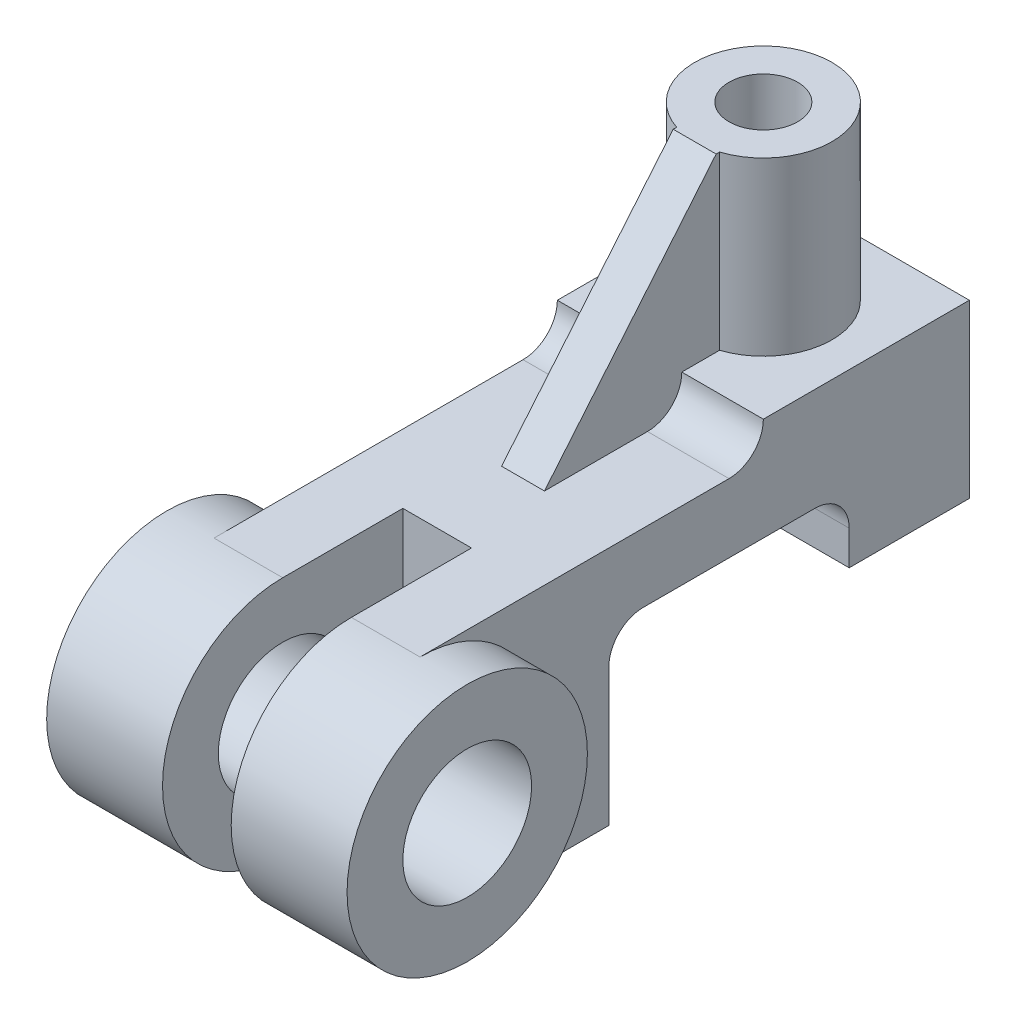
ISO-10303-21;
HEADER;
FILE_DESCRIPTION(('STEP AP214'),'2;1');
FILE_NAME('part.step','',(''),(''),'','','');
FILE_SCHEMA(('AUTOMOTIVE_DESIGN { 1 0 10303 214 1 1 1 1 }'));
ENDSEC;
DATA;
#1=APPLICATION_CONTEXT('core data for automotive mechanical design processes');
#2=APPLICATION_PROTOCOL_DEFINITION('international standard','automotive_design',2000,#1);
#3=PRODUCT_CONTEXT('',#1,'mechanical');
#4=PRODUCT('Part','Part','',(#3));
#5=PRODUCT_RELATED_PRODUCT_CATEGORY('part','',(#4));
#6=PRODUCT_DEFINITION_FORMATION('','',#4);
#7=PRODUCT_DEFINITION_CONTEXT('part definition',#1,'design');
#8=PRODUCT_DEFINITION('design','',#6,#7);
#9=PRODUCT_DEFINITION_SHAPE('','',#8);
#10=(LENGTH_UNIT() NAMED_UNIT(*) SI_UNIT(.MILLI.,.METRE.));
#11=(NAMED_UNIT(*) PLANE_ANGLE_UNIT() SI_UNIT($,.RADIAN.));
#12=(NAMED_UNIT(*) SI_UNIT($,.STERADIAN.) SOLID_ANGLE_UNIT());
#13=UNCERTAINTY_MEASURE_WITH_UNIT(LENGTH_MEASURE(1.E-05),#10,'distance_accuracy_value','');
#14=(GEOMETRIC_REPRESENTATION_CONTEXT(3) GLOBAL_UNCERTAINTY_ASSIGNED_CONTEXT((#13)) GLOBAL_UNIT_ASSIGNED_CONTEXT((#10,
#11,#12)) REPRESENTATION_CONTEXT('',''));
#15=CARTESIAN_POINT('',(0.,0.,0.));
#16=DIRECTION('',(0.,0.,1.));
#17=DIRECTION('',(1.,0.,0.));
#18=AXIS2_PLACEMENT_3D('',#15,#16,#17);
#19=CARTESIAN_POINT('',(24.,36.,-72.));
#20=DIRECTION('',(1.,0.,0.));
#21=DIRECTION('',(0.,0.,-1.));
#22=AXIS2_PLACEMENT_3D('',#19,#20,#21);
#23=CYLINDRICAL_SURFACE('',#22,8.);
#24=CARTESIAN_POINT('',(-5.,36.,-72.));
#25=DIRECTION('',(1.,0.,0.));
#26=DIRECTION('',(0.,0.,-1.));
#27=AXIS2_PLACEMENT_3D('',#24,#25,#26);
#28=CIRCLE('',#27,8.);
#29=CARTESIAN_POINT('',(-5.,36.,-80.));
#30=VERTEX_POINT('',#29);
#31=CARTESIAN_POINT('',(-5.,28.,-72.));
#32=VERTEX_POINT('',#31);
#33=EDGE_CURVE('E229',#30,#32,#28,.F.);
#34=ORIENTED_EDGE('',*,*,#33,.F.);
#35=DIRECTION('',(-1.,0.,0.));
#36=VECTOR('',#35,1.);
#37=CARTESIAN_POINT('',(24.,36.,-80.));
#38=LINE('',#37,#36);
#39=CARTESIAN_POINT('',(-24.,36.,-80.));
#40=VERTEX_POINT('',#39);
#41=EDGE_CURVE('E335',#30,#40,#38,.T.);
#42=ORIENTED_EDGE('',*,*,#41,.T.);
#43=CARTESIAN_POINT('',(-24.,36.,-72.));
#44=DIRECTION('',(1.,0.,0.));
#45=DIRECTION('',(0.,0.,-1.));
#46=AXIS2_PLACEMENT_3D('',#43,#44,#45);
#47=CIRCLE('',#46,8.);
#48=CARTESIAN_POINT('',(-24.,28.,-72.));
#49=VERTEX_POINT('',#48);
#50=EDGE_CURVE('E383',#49,#40,#47,.T.);
#51=ORIENTED_EDGE('',*,*,#50,.F.);
#52=DIRECTION('',(-1.,0.,0.));
#53=VECTOR('',#52,1.);
#54=CARTESIAN_POINT('',(-24.,28.,-72.));
#55=LINE('',#54,#53);
#56=EDGE_CURVE('E374',#32,#49,#55,.T.);
#57=ORIENTED_EDGE('',*,*,#56,.F.);
#58=EDGE_LOOP('',(#34,#42,#51,#57));
#59=FACE_BOUND('',#58,.T.);
#60=ADVANCED_FACE('F52',(#59),#23,.F.);
#61=CARTESIAN_POINT('',(35.,0.,0.));
#62=DIRECTION('',(-1.,0.,0.));
#63=DIRECTION('',(0.,0.,1.));
#64=AXIS2_PLACEMENT_3D('',#61,#62,#63);
#65=CYLINDRICAL_SURFACE('',#64,28.);
#66=CARTESIAN_POINT('',(-35.,0.,0.));
#67=DIRECTION('',(1.,0.,0.));
#68=DIRECTION('',(0.,0.,-1.));
#69=AXIS2_PLACEMENT_3D('',#66,#67,#68);
#70=CIRCLE('',#69,28.);
#71=CARTESIAN_POINT('',(-35.,0.,-28.));
#72=VERTEX_POINT('',#71);
#73=EDGE_CURVE('E355',#72,#72,#70,.T.);
#74=ORIENTED_EDGE('',*,*,#73,.T.);
#75=EDGE_LOOP('',(#74));
#76=FACE_BOUND('',#75,.T.);
#77=CARTESIAN_POINT('',(-7.99999999999999,0.,0.));
#78=DIRECTION('',(-1.,0.,0.));
#79=DIRECTION('',(0.,0.,1.));
#80=AXIS2_PLACEMENT_3D('',#77,#78,#79);
#81=CIRCLE('',#80,28.);
#82=CARTESIAN_POINT('',(-8.,-28.,0.));
#83=VERTEX_POINT('',#82);
#84=CARTESIAN_POINT('',(-8.,28.,0.));
#85=VERTEX_POINT('',#84);
#86=EDGE_CURVE('E272',#83,#85,#81,.T.);
#87=ORIENTED_EDGE('',*,*,#86,.T.);
#88=DIRECTION('',(-1.,0.,0.));
#89=VECTOR('',#88,1.);
#90=CARTESIAN_POINT('',(24.,28.,0.));
#91=LINE('',#90,#89);
#92=CARTESIAN_POINT('',(-24.,28.,0.));
#93=VERTEX_POINT('',#92);
#94=EDGE_CURVE('E303',#85,#93,#91,.T.);
#95=ORIENTED_EDGE('',*,*,#94,.T.);
#96=CARTESIAN_POINT('',(-24.,0.,0.));
#97=DIRECTION('',(1.,0.,0.));
#98=DIRECTION('',(0.,0.,-1.));
#99=AXIS2_PLACEMENT_3D('',#96,#97,#98);
#100=CIRCLE('',#99,28.);
#101=CARTESIAN_POINT('',(-24.,-28.,0.));
#102=VERTEX_POINT('',#101);
#103=EDGE_CURVE('E278',#102,#93,#100,.T.);
#104=ORIENTED_EDGE('',*,*,#103,.F.);
#105=DIRECTION('',(-1.,0.,0.));
#106=VECTOR('',#105,1.);
#107=CARTESIAN_POINT('',(24.,-28.,0.));
#108=LINE('',#107,#106);
#109=EDGE_CURVE('E345',#83,#102,#108,.T.);
#110=ORIENTED_EDGE('',*,*,#109,.F.);
#111=EDGE_LOOP('',(#87,#95,#104,#110));
#112=FACE_BOUND('',#111,.T.);
#113=ADVANCED_FACE('F422',(#76,#112),#65,.T.);
#114=CARTESIAN_POINT('',(35.,0.,0.));
#115=DIRECTION('',(-1.,0.,0.));
#116=DIRECTION('',(0.,0.,1.));
#117=AXIS2_PLACEMENT_3D('',#114,#115,#116);
#118=CYLINDRICAL_SURFACE('',#117,15.);
#119=CARTESIAN_POINT('',(-7.99999999999999,0.,0.));
#120=DIRECTION('',(-1.,0.,0.));
#121=DIRECTION('',(0.,0.,1.));
#122=AXIS2_PLACEMENT_3D('',#119,#120,#121);
#123=CIRCLE('',#122,15.);
#124=CARTESIAN_POINT('',(-7.99999999999999,0.,15.));
#125=VERTEX_POINT('',#124);
#126=EDGE_CURVE('E271',#125,#125,#123,.T.);
#127=ORIENTED_EDGE('',*,*,#126,.F.);
#128=EDGE_LOOP('',(#127));
#129=FACE_BOUND('',#128,.T.);
#130=CARTESIAN_POINT('',(-35.,0.,0.));
#131=DIRECTION('',(1.,0.,0.));
#132=DIRECTION('',(0.,0.,-1.));
#133=AXIS2_PLACEMENT_3D('',#130,#131,#132);
#134=CIRCLE('',#133,15.);
#135=CARTESIAN_POINT('',(-35.,0.,-15.));
#136=VERTEX_POINT('',#135);
#137=EDGE_CURVE('E348',#136,#136,#134,.T.);
#138=ORIENTED_EDGE('',*,*,#137,.F.);
#139=EDGE_LOOP('',(#138));
#140=FACE_BOUND('',#139,.T.);
#141=ADVANCED_FACE('F487',(#129,#140),#118,.F.);
#142=CARTESIAN_POINT('',(24.,-28.,0.));
#143=DIRECTION('',(0.,-1.,0.));
#144=DIRECTION('',(0.,0.,-1.));
#145=AXIS2_PLACEMENT_3D('',#142,#143,#144);
#146=PLANE('',#145);
#147=DIRECTION('',(-1.,0.,0.));
#148=VECTOR('',#147,1.);
#149=CARTESIAN_POINT('',(-8.,-28.,-28.));
#150=LINE('',#149,#148);
#151=CARTESIAN_POINT('',(8.,-28.,-28.));
#152=VERTEX_POINT('',#151);
#153=CARTESIAN_POINT('',(-8.,-28.,-28.));
#154=VERTEX_POINT('',#153);
#155=EDGE_CURVE('E257',#152,#154,#150,.T.);
#156=ORIENTED_EDGE('',*,*,#155,.T.);
#157=DIRECTION('',(0.,0.,1.));
#158=VECTOR('',#157,1.);
#159=CARTESIAN_POINT('',(-8.,-28.,-28.));
#160=LINE('',#159,#158);
#161=EDGE_CURVE('E252',#154,#83,#160,.T.);
#162=ORIENTED_EDGE('',*,*,#161,.T.);
#163=ORIENTED_EDGE('',*,*,#109,.T.);
#164=DIRECTION('',(0.,0.,1.));
#165=VECTOR('',#164,1.);
#166=CARTESIAN_POINT('',(-24.,-28.,0.));
#167=LINE('',#166,#165);
#168=CARTESIAN_POINT('',(-24.,-28.,-44.));
#169=VERTEX_POINT('',#168);
#170=EDGE_CURVE('E306',#169,#102,#167,.T.);
#171=ORIENTED_EDGE('',*,*,#170,.F.);
#172=DIRECTION('',(-1.,0.,0.));
#173=VECTOR('',#172,1.);
#174=CARTESIAN_POINT('',(24.,-28.,-44.));
#175=LINE('',#174,#173);
#176=CARTESIAN_POINT('',(24.,-28.,-44.));
#177=VERTEX_POINT('',#176);
#178=EDGE_CURVE('E344',#177,#169,#175,.T.);
#179=ORIENTED_EDGE('',*,*,#178,.F.);
#180=DIRECTION('',(0.,0.,1.));
#181=VECTOR('',#180,1.);
#182=CARTESIAN_POINT('',(24.,-28.,0.));
#183=LINE('',#182,#181);
#184=CARTESIAN_POINT('',(24.,-28.,0.));
#185=VERTEX_POINT('',#184);
#186=EDGE_CURVE('E280',#177,#185,#183,.T.);
#187=ORIENTED_EDGE('',*,*,#186,.T.);
#188=CARTESIAN_POINT('',(8.,-28.,0.));
#189=VERTEX_POINT('',#188);
#190=EDGE_CURVE('E341',#185,#189,#108,.T.);
#191=ORIENTED_EDGE('',*,*,#190,.T.);
#192=DIRECTION('',(0.,0.,-1.));
#193=VECTOR('',#192,1.);
#194=CARTESIAN_POINT('',(8.,-28.,-28.));
#195=LINE('',#194,#193);
#196=EDGE_CURVE('E253',#189,#152,#195,.T.);
#197=ORIENTED_EDGE('',*,*,#196,.T.);
#198=EDGE_LOOP('',(#156,#162,#163,#171,#179,#187,#191,#197));
#199=FACE_BOUND('',#198,.T.);
#200=ADVANCED_FACE('F439',(#199),#146,.T.);
#201=CARTESIAN_POINT('',(24.,28.,0.));
#202=VERTEX_POINT('',#201);
#203=CARTESIAN_POINT('',(8.,28.,0.));
#204=VERTEX_POINT('',#203);
#205=EDGE_CURVE('E329',#202,#204,#91,.T.);
#206=ORIENTED_EDGE('',*,*,#205,.T.);
#207=CARTESIAN_POINT('',(8.,0.,0.));
#208=DIRECTION('',(1.,0.,0.));
#209=DIRECTION('',(0.,0.,-1.));
#210=AXIS2_PLACEMENT_3D('',#207,#208,#209);
#211=CIRCLE('',#210,28.);
#212=EDGE_CURVE('E264',#204,#189,#211,.T.);
#213=ORIENTED_EDGE('',*,*,#212,.T.);
#214=ORIENTED_EDGE('',*,*,#190,.F.);
#215=CARTESIAN_POINT('',(24.,0.,0.));
#216=DIRECTION('',(1.,0.,0.));
#217=DIRECTION('',(0.,0.,-1.));
#218=AXIS2_PLACEMENT_3D('',#215,#216,#217);
#219=CIRCLE('',#218,28.);
#220=EDGE_CURVE('E279',#185,#202,#219,.T.);
#221=ORIENTED_EDGE('',*,*,#220,.T.);
#222=EDGE_LOOP('',(#206,#213,#214,#221));
#223=FACE_BOUND('',#222,.T.);
#224=CARTESIAN_POINT('',(35.,0.,0.));
#225=DIRECTION('',(1.,0.,0.));
#226=DIRECTION('',(0.,0.,-1.));
#227=AXIS2_PLACEMENT_3D('',#224,#225,#226);
#228=CIRCLE('',#227,28.);
#229=CARTESIAN_POINT('',(35.,0.,-28.));
#230=VERTEX_POINT('',#229);
#231=EDGE_CURVE('E354',#230,#230,#228,.T.);
#232=ORIENTED_EDGE('',*,*,#231,.F.);
#233=EDGE_LOOP('',(#232));
#234=FACE_BOUND('',#233,.T.);
#235=ADVANCED_FACE('F433',(#223,#234),#65,.T.);
#236=CARTESIAN_POINT('',(35.,0.,0.));
#237=DIRECTION('',(1.,0.,0.));
#238=DIRECTION('',(0.,0.,-1.));
#239=AXIS2_PLACEMENT_3D('',#236,#237,#238);
#240=PLANE('',#239);
#241=ORIENTED_EDGE('',*,*,#231,.T.);
#242=EDGE_LOOP('',(#241));
#243=FACE_BOUND('',#242,.T.);
#244=CARTESIAN_POINT('',(35.,0.,0.));
#245=DIRECTION('',(1.,0.,0.));
#246=DIRECTION('',(0.,0.,-1.));
#247=AXIS2_PLACEMENT_3D('',#244,#245,#246);
#248=CIRCLE('',#247,15.);
#249=CARTESIAN_POINT('',(35.,0.,-15.));
#250=VERTEX_POINT('',#249);
#251=EDGE_CURVE('E349',#250,#250,#248,.T.);
#252=ORIENTED_EDGE('',*,*,#251,.F.);
#253=EDGE_LOOP('',(#252));
#254=FACE_BOUND('',#253,.T.);
#255=ADVANCED_FACE('F503',(#243,#254),#240,.T.);
#256=CARTESIAN_POINT('',(-35.,0.,0.));
#257=DIRECTION('',(1.,0.,0.));
#258=DIRECTION('',(0.,0.,-1.));
#259=AXIS2_PLACEMENT_3D('',#256,#257,#258);
#260=PLANE('',#259);
#261=ORIENTED_EDGE('',*,*,#73,.F.);
#262=EDGE_LOOP('',(#261));
#263=FACE_BOUND('',#262,.T.);
#264=ORIENTED_EDGE('',*,*,#137,.T.);
#265=EDGE_LOOP('',(#264));
#266=FACE_BOUND('',#265,.T.);
#267=ADVANCED_FACE('F502',(#263,#266),#260,.F.);
#268=CARTESIAN_POINT('',(8.,0.,0.));
#269=DIRECTION('',(1.,0.,0.));
#270=DIRECTION('',(0.,0.,-1.));
#271=AXIS2_PLACEMENT_3D('',#268,#269,#270);
#272=CIRCLE('',#271,15.);
#273=CARTESIAN_POINT('',(8.,0.,-15.));
#274=VERTEX_POINT('',#273);
#275=EDGE_CURVE('E267',#274,#274,#272,.T.);
#276=ORIENTED_EDGE('',*,*,#275,.F.);
#277=EDGE_LOOP('',(#276));
#278=FACE_BOUND('',#277,.T.);
#279=ORIENTED_EDGE('',*,*,#251,.T.);
#280=EDGE_LOOP('',(#279));
#281=FACE_BOUND('',#280,.T.);
#282=ADVANCED_FACE('F510',(#278,#281),#118,.F.);
#283=CARTESIAN_POINT('',(24.,0.,-44.));
#284=DIRECTION('',(0.,0.,-1.));
#285=DIRECTION('',(0.,1.,0.));
#286=AXIS2_PLACEMENT_3D('',#283,#284,#285);
#287=PLANE('',#286);
#288=ORIENTED_EDGE('',*,*,#178,.T.);
#289=DIRECTION('',(0.,-1.,0.));
#290=VECTOR('',#289,1.);
#291=CARTESIAN_POINT('',(-24.,0.,-44.));
#292=LINE('',#291,#290);
#293=CARTESIAN_POINT('',(-24.,3.99999999999999,-44.));
#294=VERTEX_POINT('',#293);
#295=EDGE_CURVE('E307',#294,#169,#292,.T.);
#296=ORIENTED_EDGE('',*,*,#295,.F.);
#297=DIRECTION('',(-1.,0.,0.));
#298=VECTOR('',#297,1.);
#299=CARTESIAN_POINT('',(24.,3.99999999999999,-44.));
#300=LINE('',#299,#298);
#301=CARTESIAN_POINT('',(24.,3.99999999999999,-44.));
#302=VERTEX_POINT('',#301);
#303=EDGE_CURVE('E373',#294,#302,#300,.F.);
#304=ORIENTED_EDGE('',*,*,#303,.T.);
#305=DIRECTION('',(0.,-1.,0.));
#306=VECTOR('',#305,1.);
#307=CARTESIAN_POINT('',(24.,0.,-44.));
#308=LINE('',#307,#306);
#309=EDGE_CURVE('E283',#302,#177,#308,.T.);
#310=ORIENTED_EDGE('',*,*,#309,.T.);
#311=EDGE_LOOP('',(#288,#296,#304,#310));
#312=FACE_BOUND('',#311,.T.);
#313=ADVANCED_FACE('F443',(#312),#287,.T.);
#314=CARTESIAN_POINT('',(24.,12.,0.));
#315=DIRECTION('',(0.,-1.,0.));
#316=DIRECTION('',(0.,0.,-1.));
#317=AXIS2_PLACEMENT_3D('',#314,#315,#316);
#318=PLANE('',#317);
#319=DIRECTION('',(-1.,0.,0.));
#320=VECTOR('',#319,1.);
#321=CARTESIAN_POINT('',(-24.,12.,-52.));
#322=LINE('',#321,#320);
#323=CARTESIAN_POINT('',(24.,12.,-52.));
#324=VERTEX_POINT('',#323);
#325=CARTESIAN_POINT('',(-24.,12.,-52.));
#326=VERTEX_POINT('',#325);
#327=EDGE_CURVE('E367',#324,#326,#322,.T.);
#328=ORIENTED_EDGE('',*,*,#327,.T.);
#329=DIRECTION('',(0.,0.,1.));
#330=VECTOR('',#329,1.);
#331=CARTESIAN_POINT('',(-24.,12.,0.));
#332=LINE('',#331,#330);
#333=CARTESIAN_POINT('',(-24.,12.,-92.));
#334=VERTEX_POINT('',#333);
#335=EDGE_CURVE('E315',#334,#326,#332,.T.);
#336=ORIENTED_EDGE('',*,*,#335,.F.);
#337=DIRECTION('',(-1.,0.,0.));
#338=VECTOR('',#337,1.);
#339=CARTESIAN_POINT('',(24.,12.,-92.));
#340=LINE('',#339,#338);
#341=CARTESIAN_POINT('',(24.,12.,-92.));
#342=VERTEX_POINT('',#341);
#343=EDGE_CURVE('E371',#334,#342,#340,.F.);
#344=ORIENTED_EDGE('',*,*,#343,.T.);
#345=DIRECTION('',(0.,0.,1.));
#346=VECTOR('',#345,1.);
#347=CARTESIAN_POINT('',(24.,12.,0.));
#348=LINE('',#347,#346);
#349=EDGE_CURVE('E281',#342,#324,#348,.T.);
#350=ORIENTED_EDGE('',*,*,#349,.T.);
#351=EDGE_LOOP('',(#328,#336,#344,#350));
#352=FACE_BOUND('',#351,.T.);
#353=ADVANCED_FACE('F451',(#352),#318,.T.);
#354=CARTESIAN_POINT('',(24.,0.,-100.));
#355=DIRECTION('',(0.,0.,1.));
#356=DIRECTION('',(1.,0.,0.));
#357=AXIS2_PLACEMENT_3D('',#354,#355,#356);
#358=PLANE('',#357);
#359=DIRECTION('',(-1.,0.,0.));
#360=VECTOR('',#359,1.);
#361=CARTESIAN_POINT('',(-24.,4.,-100.));
#362=LINE('',#361,#360);
#363=CARTESIAN_POINT('',(24.,4.,-100.));
#364=VERTEX_POINT('',#363);
#365=CARTESIAN_POINT('',(-24.,4.,-100.));
#366=VERTEX_POINT('',#365);
#367=EDGE_CURVE('E370',#364,#366,#362,.T.);
#368=ORIENTED_EDGE('',*,*,#367,.T.);
#369=DIRECTION('',(0.,1.,0.));
#370=VECTOR('',#369,1.);
#371=CARTESIAN_POINT('',(-24.,0.,-100.));
#372=LINE('',#371,#370);
#373=CARTESIAN_POINT('',(-24.,-4.,-100.));
#374=VERTEX_POINT('',#373);
#375=EDGE_CURVE('E314',#374,#366,#372,.T.);
#376=ORIENTED_EDGE('',*,*,#375,.F.);
#377=DIRECTION('',(-1.,0.,0.));
#378=VECTOR('',#377,1.);
#379=CARTESIAN_POINT('',(24.,-4.,-100.));
#380=LINE('',#379,#378);
#381=CARTESIAN_POINT('',(24.,-4.,-100.));
#382=VERTEX_POINT('',#381);
#383=EDGE_CURVE('E338',#382,#374,#380,.T.);
#384=ORIENTED_EDGE('',*,*,#383,.F.);
#385=DIRECTION('',(0.,1.,0.));
#386=VECTOR('',#385,1.);
#387=CARTESIAN_POINT('',(24.,0.,-100.));
#388=LINE('',#387,#386);
#389=EDGE_CURVE('E287',#382,#364,#388,.T.);
#390=ORIENTED_EDGE('',*,*,#389,.T.);
#391=EDGE_LOOP('',(#368,#376,#384,#390));
#392=FACE_BOUND('',#391,.T.);
#393=ADVANCED_FACE('F463',(#392),#358,.T.);
#394=CARTESIAN_POINT('',(24.,-4.00000000000001,0.));
#395=DIRECTION('',(0.,-1.,0.));
#396=DIRECTION('',(0.,0.,-1.));
#397=AXIS2_PLACEMENT_3D('',#394,#395,#396);
#398=PLANE('',#397);
#399=ORIENTED_EDGE('',*,*,#383,.T.);
#400=DIRECTION('',(0.,0.,1.));
#401=VECTOR('',#400,1.);
#402=CARTESIAN_POINT('',(-24.,-4.00000000000001,0.));
#403=LINE('',#402,#401);
#404=CARTESIAN_POINT('',(-24.,-4.,-128.));
#405=VERTEX_POINT('',#404);
#406=EDGE_CURVE('E319',#405,#374,#403,.T.);
#407=ORIENTED_EDGE('',*,*,#406,.F.);
#408=DIRECTION('',(-1.,0.,0.));
#409=VECTOR('',#408,1.);
#410=CARTESIAN_POINT('',(24.,-4.,-128.));
#411=LINE('',#410,#409);
#412=CARTESIAN_POINT('',(24.,-4.,-128.));
#413=VERTEX_POINT('',#412);
#414=EDGE_CURVE('E336',#413,#405,#411,.T.);
#415=ORIENTED_EDGE('',*,*,#414,.F.);
#416=DIRECTION('',(0.,0.,1.));
#417=VECTOR('',#416,1.);
#418=CARTESIAN_POINT('',(24.,-4.00000000000001,0.));
#419=LINE('',#418,#417);
#420=EDGE_CURVE('E293',#413,#382,#419,.T.);
#421=ORIENTED_EDGE('',*,*,#420,.T.);
#422=EDGE_LOOP('',(#399,#407,#415,#421));
#423=FACE_BOUND('',#422,.T.);
#424=ADVANCED_FACE('F466',(#423),#398,.T.);
#425=CARTESIAN_POINT('',(24.,0.,-128.));
#426=DIRECTION('',(0.,0.,-1.));
#427=DIRECTION('',(-1.,0.,0.));
#428=AXIS2_PLACEMENT_3D('',#425,#426,#427);
#429=PLANE('',#428);
#430=ORIENTED_EDGE('',*,*,#414,.T.);
#431=DIRECTION('',(0.,-1.,0.));
#432=VECTOR('',#431,1.);
#433=CARTESIAN_POINT('',(-24.,0.,-128.));
#434=LINE('',#433,#432);
#435=CARTESIAN_POINT('',(-24.,36.,-128.));
#436=VERTEX_POINT('',#435);
#437=EDGE_CURVE('E323',#436,#405,#434,.T.);
#438=ORIENTED_EDGE('',*,*,#437,.F.);
#439=DIRECTION('',(-1.,0.,0.));
#440=VECTOR('',#439,1.);
#441=CARTESIAN_POINT('',(24.,36.,-128.));
#442=LINE('',#441,#440);
#443=CARTESIAN_POINT('',(24.,36.,-128.));
#444=VERTEX_POINT('',#443);
#445=EDGE_CURVE('E337',#444,#436,#442,.T.);
#446=ORIENTED_EDGE('',*,*,#445,.F.);
#447=DIRECTION('',(0.,-1.,0.));
#448=VECTOR('',#447,1.);
#449=CARTESIAN_POINT('',(24.,0.,-128.));
#450=LINE('',#449,#448);
#451=EDGE_CURVE('E295',#444,#413,#450,.T.);
#452=ORIENTED_EDGE('',*,*,#451,.T.);
#453=EDGE_LOOP('',(#430,#438,#446,#452));
#454=FACE_BOUND('',#453,.T.);
#455=ADVANCED_FACE('F468',(#454),#429,.T.);
#456=CARTESIAN_POINT('',(24.,36.,0.));
#457=DIRECTION('',(0.,1.,0.));
#458=DIRECTION('',(0.,0.,1.));
#459=AXIS2_PLACEMENT_3D('',#456,#457,#458);
#460=PLANE('',#459);
#461=DIRECTION('',(0.,0.,-1.));
#462=VECTOR('',#461,1.);
#463=CARTESIAN_POINT('',(5.,36.,0.));
#464=LINE('',#463,#462);
#465=CARTESIAN_POINT('',(5.,36.,-80.));
#466=VERTEX_POINT('',#465);
#467=CARTESIAN_POINT('',(5.,36.,-88.8013158464293));
#468=VERTEX_POINT('',#467);
#469=EDGE_CURVE('E240',#466,#468,#464,.T.);
#470=ORIENTED_EDGE('',*,*,#469,.F.);
#471=CARTESIAN_POINT('',(24.,36.,-80.));
#472=VERTEX_POINT('',#471);
#473=EDGE_CURVE('E332',#472,#466,#38,.T.);
#474=ORIENTED_EDGE('',*,*,#473,.F.);
#475=DIRECTION('',(0.,0.,-1.));
#476=VECTOR('',#475,1.);
#477=CARTESIAN_POINT('',(24.,36.,0.));
#478=LINE('',#477,#476);
#479=EDGE_CURVE('E300',#472,#444,#478,.T.);
#480=ORIENTED_EDGE('',*,*,#479,.T.);
#481=ORIENTED_EDGE('',*,*,#445,.T.);
#482=DIRECTION('',(0.,0.,-1.));
#483=VECTOR('',#482,1.);
#484=CARTESIAN_POINT('',(-24.,36.,0.));
#485=LINE('',#484,#483);
#486=EDGE_CURVE('E325',#40,#436,#485,.T.);
#487=ORIENTED_EDGE('',*,*,#486,.F.);
#488=ORIENTED_EDGE('',*,*,#41,.F.);
#489=DIRECTION('',(0.,0.,-1.));
#490=VECTOR('',#489,1.);
#491=CARTESIAN_POINT('',(-5.,36.,0.));
#492=LINE('',#491,#490);
#493=CARTESIAN_POINT('',(-5.,36.,-88.8013158464293));
#494=VERTEX_POINT('',#493);
#495=EDGE_CURVE('E227',#30,#494,#492,.T.);
#496=ORIENTED_EDGE('',*,*,#495,.T.);
#497=CARTESIAN_POINT('',(0.,36.,-104.));
#498=DIRECTION('',(0.,1.,0.));
#499=DIRECTION('',(0.,0.,1.));
#500=AXIS2_PLACEMENT_3D('',#497,#498,#499);
#501=CIRCLE('',#500,16.);
#502=EDGE_CURVE('E12',#468,#494,#501,.T.);
#503=ORIENTED_EDGE('',*,*,#502,.F.);
#504=EDGE_LOOP('',(#470,#474,#480,#481,#487,#488,#496,#503));
#505=FACE_BOUND('',#504,.T.);
#506=ADVANCED_FACE('F403',(#505),#460,.T.);
#507=CARTESIAN_POINT('',(24.,28.,0.));
#508=DIRECTION('',(0.,1.,0.));
#509=DIRECTION('',(0.,0.,1.));
#510=AXIS2_PLACEMENT_3D('',#507,#508,#509);
#511=PLANE('',#510);
#512=DIRECTION('',(0.,0.,-1.));
#513=VECTOR('',#512,1.);
#514=CARTESIAN_POINT('',(5.,28.,0.));
#515=LINE('',#514,#513);
#516=CARTESIAN_POINT('',(5.,28.,-48.));
#517=VERTEX_POINT('',#516);
#518=CARTESIAN_POINT('',(5.,28.,-72.));
#519=VERTEX_POINT('',#518);
#520=EDGE_CURVE('E69',#517,#519,#515,.T.);
#521=ORIENTED_EDGE('',*,*,#520,.F.);
#522=DIRECTION('',(1.,0.,0.));
#523=VECTOR('',#522,1.);
#524=CARTESIAN_POINT('',(24.,28.,-48.));
#525=LINE('',#524,#523);
#526=CARTESIAN_POINT('',(-5.,28.,-48.));
#527=VERTEX_POINT('',#526);
#528=EDGE_CURVE('E72',#527,#517,#525,.T.);
#529=ORIENTED_EDGE('',*,*,#528,.F.);
#530=DIRECTION('',(0.,0.,-1.));
#531=VECTOR('',#530,1.);
#532=CARTESIAN_POINT('',(-5.,28.,0.));
#533=LINE('',#532,#531);
#534=EDGE_CURVE('E232',#527,#32,#533,.T.);
#535=ORIENTED_EDGE('',*,*,#534,.T.);
#536=ORIENTED_EDGE('',*,*,#56,.T.);
#537=DIRECTION('',(0.,0.,-1.));
#538=VECTOR('',#537,1.);
#539=CARTESIAN_POINT('',(-24.,28.,0.));
#540=LINE('',#539,#538);
#541=EDGE_CURVE('E276',#93,#49,#540,.T.);
#542=ORIENTED_EDGE('',*,*,#541,.F.);
#543=ORIENTED_EDGE('',*,*,#94,.F.);
#544=DIRECTION('',(0.,0.,1.));
#545=VECTOR('',#544,1.);
#546=CARTESIAN_POINT('',(-8.,28.,0.));
#547=LINE('',#546,#545);
#548=CARTESIAN_POINT('',(-8.,28.,-28.));
#549=VERTEX_POINT('',#548);
#550=EDGE_CURVE('E364',#549,#85,#547,.T.);
#551=ORIENTED_EDGE('',*,*,#550,.F.);
#552=DIRECTION('',(-1.,0.,0.));
#553=VECTOR('',#552,1.);
#554=CARTESIAN_POINT('',(24.,28.,-28.));
#555=LINE('',#554,#553);
#556=CARTESIAN_POINT('',(8.,28.,-28.));
#557=VERTEX_POINT('',#556);
#558=EDGE_CURVE('E365',#557,#549,#555,.T.);
#559=ORIENTED_EDGE('',*,*,#558,.F.);
#560=DIRECTION('',(0.,0.,-1.));
#561=VECTOR('',#560,1.);
#562=CARTESIAN_POINT('',(8.,28.,0.));
#563=LINE('',#562,#561);
#564=EDGE_CURVE('E356',#204,#557,#563,.T.);
#565=ORIENTED_EDGE('',*,*,#564,.F.);
#566=ORIENTED_EDGE('',*,*,#205,.F.);
#567=DIRECTION('',(0.,0.,-1.));
#568=VECTOR('',#567,1.);
#569=CARTESIAN_POINT('',(24.,28.,0.));
#570=LINE('',#569,#568);
#571=CARTESIAN_POINT('',(24.,28.,-72.));
#572=VERTEX_POINT('',#571);
#573=EDGE_CURVE('E297',#202,#572,#570,.T.);
#574=ORIENTED_EDGE('',*,*,#573,.T.);
#575=EDGE_CURVE('E376',#572,#519,#55,.T.);
#576=ORIENTED_EDGE('',*,*,#575,.T.);
#577=EDGE_LOOP('',(#521,#529,#535,#536,#542,#543,#551,#559,#565,#566,#574,#576));
#578=FACE_BOUND('',#577,.T.);
#579=ADVANCED_FACE('F399',(#578),#511,.T.);
#580=CARTESIAN_POINT('',(24.,0.,0.));
#581=DIRECTION('',(1.,0.,0.));
#582=DIRECTION('',(0.,0.,-1.));
#583=AXIS2_PLACEMENT_3D('',#580,#581,#582);
#584=PLANE('',#583);
#585=ORIENTED_EDGE('',*,*,#220,.F.);
#586=ORIENTED_EDGE('',*,*,#186,.F.);
#587=ORIENTED_EDGE('',*,*,#309,.F.);
#588=CARTESIAN_POINT('',(24.,4.,-52.));
#589=DIRECTION('',(1.,0.,0.));
#590=DIRECTION('',(0.,0.,-1.));
#591=AXIS2_PLACEMENT_3D('',#588,#589,#590);
#592=CIRCLE('',#591,8.);
#593=EDGE_CURVE('E381',#302,#324,#592,.F.);
#594=ORIENTED_EDGE('',*,*,#593,.T.);
#595=ORIENTED_EDGE('',*,*,#349,.F.);
#596=CARTESIAN_POINT('',(24.,4.,-92.));
#597=DIRECTION('',(1.,0.,0.));
#598=DIRECTION('',(0.,0.,-1.));
#599=AXIS2_PLACEMENT_3D('',#596,#597,#598);
#600=CIRCLE('',#599,8.);
#601=EDGE_CURVE('E379',#342,#364,#600,.F.);
#602=ORIENTED_EDGE('',*,*,#601,.T.);
#603=ORIENTED_EDGE('',*,*,#389,.F.);
#604=ORIENTED_EDGE('',*,*,#420,.F.);
#605=ORIENTED_EDGE('',*,*,#451,.F.);
#606=ORIENTED_EDGE('',*,*,#479,.F.);
#607=CARTESIAN_POINT('',(24.,36.,-72.));
#608=DIRECTION('',(1.,0.,0.));
#609=DIRECTION('',(0.,0.,-1.));
#610=AXIS2_PLACEMENT_3D('',#607,#608,#609);
#611=CIRCLE('',#610,8.);
#612=EDGE_CURVE('E60',#472,#572,#611,.F.);
#613=ORIENTED_EDGE('',*,*,#612,.T.);
#614=ORIENTED_EDGE('',*,*,#573,.F.);
#615=EDGE_LOOP('',(#585,#586,#587,#594,#595,#602,#603,#604,#605,#606,#613,#614));
#616=FACE_BOUND('',#615,.T.);
#617=ADVANCED_FACE('F391',(#616),#584,.T.);
#618=CARTESIAN_POINT('',(-24.,0.,0.));
#619=DIRECTION('',(1.,0.,0.));
#620=DIRECTION('',(0.,0.,-1.));
#621=AXIS2_PLACEMENT_3D('',#618,#619,#620);
#622=PLANE('',#621);
#623=ORIENTED_EDGE('',*,*,#103,.T.);
#624=ORIENTED_EDGE('',*,*,#541,.T.);
#625=ORIENTED_EDGE('',*,*,#50,.T.);
#626=ORIENTED_EDGE('',*,*,#486,.T.);
#627=ORIENTED_EDGE('',*,*,#437,.T.);
#628=ORIENTED_EDGE('',*,*,#406,.T.);
#629=ORIENTED_EDGE('',*,*,#375,.T.);
#630=CARTESIAN_POINT('',(-24.,4.,-92.));
#631=DIRECTION('',(1.,0.,0.));
#632=DIRECTION('',(0.,0.,-1.));
#633=AXIS2_PLACEMENT_3D('',#630,#631,#632);
#634=CIRCLE('',#633,8.);
#635=EDGE_CURVE('E377',#366,#334,#634,.T.);
#636=ORIENTED_EDGE('',*,*,#635,.T.);
#637=ORIENTED_EDGE('',*,*,#335,.T.);
#638=CARTESIAN_POINT('',(-24.,4.,-52.));
#639=DIRECTION('',(1.,0.,0.));
#640=DIRECTION('',(0.,0.,-1.));
#641=AXIS2_PLACEMENT_3D('',#638,#639,#640);
#642=CIRCLE('',#641,8.);
#643=EDGE_CURVE('E385',#326,#294,#642,.T.);
#644=ORIENTED_EDGE('',*,*,#643,.T.);
#645=ORIENTED_EDGE('',*,*,#295,.T.);
#646=ORIENTED_EDGE('',*,*,#170,.T.);
#647=EDGE_LOOP('',(#623,#624,#625,#626,#627,#628,#629,#636,#637,#644,#645,#646));
#648=FACE_BOUND('',#647,.T.);
#649=ADVANCED_FACE('F416',(#648),#622,.F.);
#650=CARTESIAN_POINT('',(-8.,-28.,-28.));
#651=DIRECTION('',(-1.,0.,0.));
#652=DIRECTION('',(0.,0.,1.));
#653=AXIS2_PLACEMENT_3D('',#650,#651,#652);
#654=PLANE('',#653);
#655=ORIENTED_EDGE('',*,*,#126,.T.);
#656=EDGE_LOOP('',(#655));
#657=FACE_BOUND('',#656,.T.);
#658=ORIENTED_EDGE('',*,*,#161,.F.);
#659=DIRECTION('',(0.,1.,0.));
#660=VECTOR('',#659,1.);
#661=CARTESIAN_POINT('',(-8.,-28.,-28.));
#662=LINE('',#661,#660);
#663=EDGE_CURVE('E262',#154,#549,#662,.T.);
#664=ORIENTED_EDGE('',*,*,#663,.T.);
#665=ORIENTED_EDGE('',*,*,#550,.T.);
#666=ORIENTED_EDGE('',*,*,#86,.F.);
#667=EDGE_LOOP('',(#658,#664,#665,#666));
#668=FACE_BOUND('',#667,.T.);
#669=ADVANCED_FACE('F428',(#657,#668),#654,.F.);
#670=CARTESIAN_POINT('',(8.,-28.,-28.));
#671=DIRECTION('',(1.,0.,0.));
#672=DIRECTION('',(0.,0.,-1.));
#673=AXIS2_PLACEMENT_3D('',#670,#671,#672);
#674=PLANE('',#673);
#675=ORIENTED_EDGE('',*,*,#275,.T.);
#676=EDGE_LOOP('',(#675));
#677=FACE_BOUND('',#676,.T.);
#678=ORIENTED_EDGE('',*,*,#212,.F.);
#679=ORIENTED_EDGE('',*,*,#564,.T.);
#680=DIRECTION('',(0.,1.,0.));
#681=VECTOR('',#680,1.);
#682=CARTESIAN_POINT('',(8.,-28.,-28.));
#683=LINE('',#682,#681);
#684=EDGE_CURVE('E256',#152,#557,#683,.T.);
#685=ORIENTED_EDGE('',*,*,#684,.F.);
#686=ORIENTED_EDGE('',*,*,#196,.F.);
#687=EDGE_LOOP('',(#678,#679,#685,#686));
#688=FACE_BOUND('',#687,.T.);
#689=ADVANCED_FACE('F593',(#677,#688),#674,.F.);
#690=CARTESIAN_POINT('',(-8.,-28.,-28.));
#691=DIRECTION('',(0.,0.,-1.));
#692=DIRECTION('',(-1.,0.,0.));
#693=AXIS2_PLACEMENT_3D('',#690,#691,#692);
#694=PLANE('',#693);
#695=ORIENTED_EDGE('',*,*,#663,.F.);
#696=ORIENTED_EDGE('',*,*,#155,.F.);
#697=ORIENTED_EDGE('',*,*,#684,.T.);
#698=ORIENTED_EDGE('',*,*,#558,.T.);
#699=EDGE_LOOP('',(#695,#696,#697,#698));
#700=FACE_BOUND('',#699,.T.);
#701=ADVANCED_FACE('F427',(#700),#694,.F.);
#702=CARTESIAN_POINT('',(24.,4.,-92.));
#703=DIRECTION('',(1.,0.,0.));
#704=DIRECTION('',(0.,0.,-1.));
#705=AXIS2_PLACEMENT_3D('',#702,#703,#704);
#706=CYLINDRICAL_SURFACE('',#705,8.);
#707=ORIENTED_EDGE('',*,*,#601,.F.);
#708=ORIENTED_EDGE('',*,*,#343,.F.);
#709=ORIENTED_EDGE('',*,*,#635,.F.);
#710=ORIENTED_EDGE('',*,*,#367,.F.);
#711=EDGE_LOOP('',(#707,#708,#709,#710));
#712=FACE_BOUND('',#711,.T.);
#713=ADVANCED_FACE('F459',(#712),#706,.F.);
#714=CARTESIAN_POINT('',(24.,4.,-52.));
#715=DIRECTION('',(1.,0.,0.));
#716=DIRECTION('',(0.,0.,-1.));
#717=AXIS2_PLACEMENT_3D('',#714,#715,#716);
#718=CYLINDRICAL_SURFACE('',#717,8.);
#719=ORIENTED_EDGE('',*,*,#593,.F.);
#720=ORIENTED_EDGE('',*,*,#303,.F.);
#721=ORIENTED_EDGE('',*,*,#643,.F.);
#722=ORIENTED_EDGE('',*,*,#327,.F.);
#723=EDGE_LOOP('',(#719,#720,#721,#722));
#724=FACE_BOUND('',#723,.T.);
#725=ADVANCED_FACE('F453',(#724),#718,.F.);
#726=ORIENTED_EDGE('',*,*,#473,.T.);
#727=CARTESIAN_POINT('',(5.,36.,-72.));
#728=DIRECTION('',(1.,0.,0.));
#729=DIRECTION('',(0.,0.,-1.));
#730=AXIS2_PLACEMENT_3D('',#727,#728,#729);
#731=CIRCLE('',#730,8.);
#732=EDGE_CURVE('E237',#466,#519,#731,.F.);
#733=ORIENTED_EDGE('',*,*,#732,.T.);
#734=ORIENTED_EDGE('',*,*,#575,.F.);
#735=ORIENTED_EDGE('',*,*,#612,.F.);
#736=EDGE_LOOP('',(#726,#733,#734,#735));
#737=FACE_BOUND('',#736,.T.);
#738=ADVANCED_FACE('F54',(#737),#23,.F.);
#739=CARTESIAN_POINT('',(0.,76.,-104.));
#740=DIRECTION('',(0.,1.,0.));
#741=DIRECTION('',(0.,0.,1.));
#742=AXIS2_PLACEMENT_3D('',#739,#740,#741);
#743=PLANE('',#742);
#744=CARTESIAN_POINT('',(0.,76.,-104.));
#745=DIRECTION('',(0.,1.,0.));
#746=DIRECTION('',(0.,0.,1.));
#747=AXIS2_PLACEMENT_3D('',#744,#745,#746);
#748=CIRCLE('',#747,8.);
#749=CARTESIAN_POINT('',(0.,76.,-96.));
#750=VERTEX_POINT('',#749);
#751=EDGE_CURVE('E244',#750,#750,#748,.T.);
#752=ORIENTED_EDGE('',*,*,#751,.F.);
#753=EDGE_LOOP('',(#752));
#754=FACE_BOUND('',#753,.T.);
#755=DIRECTION('',(0.,0.,-1.));
#756=VECTOR('',#755,1.);
#757=CARTESIAN_POINT('',(5.,76.,-50.));
#758=LINE('',#757,#756);
#759=CARTESIAN_POINT('',(5.,76.,-88.8013158464293));
#760=VERTEX_POINT('',#759);
#761=CARTESIAN_POINT('',(5.,76.,-87.9999));
#762=VERTEX_POINT('',#761);
#763=EDGE_CURVE('E205',#760,#762,#758,.F.);
#764=ORIENTED_EDGE('',*,*,#763,.F.);
#765=CARTESIAN_POINT('',(0.,76.,-104.));
#766=DIRECTION('',(0.,1.,0.));
#767=DIRECTION('',(0.,0.,1.));
#768=AXIS2_PLACEMENT_3D('',#765,#766,#767);
#769=CIRCLE('',#768,16.);
#770=CARTESIAN_POINT('',(-5.,76.,-88.8013158464293));
#771=VERTEX_POINT('',#770);
#772=EDGE_CURVE('E247',#760,#771,#769,.T.);
#773=ORIENTED_EDGE('',*,*,#772,.T.);
#774=DIRECTION('',(0.,0.,-1.));
#775=VECTOR('',#774,1.);
#776=CARTESIAN_POINT('',(-5.,76.,-50.));
#777=LINE('',#776,#775);
#778=CARTESIAN_POINT('',(-5.,76.,-87.9999));
#779=VERTEX_POINT('',#778);
#780=EDGE_CURVE('E217',#771,#779,#777,.F.);
#781=ORIENTED_EDGE('',*,*,#780,.T.);
#782=DIRECTION('',(1.,0.,0.));
#783=VECTOR('',#782,1.);
#784=CARTESIAN_POINT('',(0.,76.,-87.9999));
#785=LINE('',#784,#783);
#786=EDGE_CURVE('E212',#779,#762,#785,.T.);
#787=ORIENTED_EDGE('',*,*,#786,.T.);
#788=EDGE_LOOP('',(#764,#773,#781,#787));
#789=FACE_BOUND('',#788,.T.);
#790=ADVANCED_FACE('F215',(#754,#789),#743,.T.);
#791=CARTESIAN_POINT('',(0.,76.,-104.));
#792=DIRECTION('',(0.,-1.,0.));
#793=DIRECTION('',(0.,0.,-1.));
#794=AXIS2_PLACEMENT_3D('',#791,#792,#793);
#795=CYLINDRICAL_SURFACE('',#794,16.);
#796=ORIENTED_EDGE('',*,*,#772,.F.);
#797=DIRECTION('',(0.,-1.,0.));
#798=VECTOR('',#797,1.);
#799=CARTESIAN_POINT('',(5.,76.,-88.8013158464293));
#800=LINE('',#799,#798);
#801=EDGE_CURVE('E206',#760,#468,#800,.T.);
#802=ORIENTED_EDGE('',*,*,#801,.T.);
#803=ORIENTED_EDGE('',*,*,#502,.T.);
#804=DIRECTION('',(0.,-1.,0.));
#805=VECTOR('',#804,1.);
#806=CARTESIAN_POINT('',(-5.,76.,-88.8013158464293));
#807=LINE('',#806,#805);
#808=EDGE_CURVE('E216',#771,#494,#807,.T.);
#809=ORIENTED_EDGE('',*,*,#808,.F.);
#810=EDGE_LOOP('',(#796,#802,#803,#809));
#811=FACE_BOUND('',#810,.T.);
#812=ADVANCED_FACE('F406',(#811),#795,.T.);
#813=CARTESIAN_POINT('',(0.,76.,-104.));
#814=DIRECTION('',(0.,-1.,0.));
#815=DIRECTION('',(0.,0.,-1.));
#816=AXIS2_PLACEMENT_3D('',#813,#814,#815);
#817=CYLINDRICAL_SURFACE('',#816,8.);
#818=CARTESIAN_POINT('',(0.,36.,-104.));
#819=DIRECTION('',(0.,1.,0.));
#820=DIRECTION('',(0.,0.,1.));
#821=AXIS2_PLACEMENT_3D('',#818,#819,#820);
#822=CIRCLE('',#821,8.);
#823=CARTESIAN_POINT('',(0.,36.,-96.));
#824=VERTEX_POINT('',#823);
#825=EDGE_CURVE('E242',#824,#824,#822,.T.);
#826=ORIENTED_EDGE('',*,*,#825,.F.);
#827=EDGE_LOOP('',(#826));
#828=FACE_BOUND('',#827,.T.);
#829=ORIENTED_EDGE('',*,*,#751,.T.);
#830=EDGE_LOOP('',(#829));
#831=FACE_BOUND('',#830,.T.);
#832=ADVANCED_FACE('F632',(#828,#831),#817,.F.);
#833=ORIENTED_EDGE('',*,*,#825,.T.);
#834=EDGE_LOOP('',(#833));
#835=FACE_BOUND('',#834,.T.);
#836=ADVANCED_FACE('F479',(#835),#460,.T.);
#837=CARTESIAN_POINT('',(5.,24.,-50.));
#838=DIRECTION('',(1.,0.,0.));
#839=DIRECTION('',(0.,0.,-1.));
#840=AXIS2_PLACEMENT_3D('',#837,#838,#839);
#841=PLANE('',#840);
#842=DIRECTION('',(0.,-0.768222066709568,0.640183455128668));
#843=VECTOR('',#842,1.);
#844=CARTESIAN_POINT('',(5.,76.,-87.9999));
#845=LINE('',#844,#843);
#846=EDGE_CURVE('E207',#762,#517,#845,.T.);
#847=ORIENTED_EDGE('',*,*,#846,.T.);
#848=ORIENTED_EDGE('',*,*,#520,.T.);
#849=ORIENTED_EDGE('',*,*,#732,.F.);
#850=ORIENTED_EDGE('',*,*,#469,.T.);
#851=ORIENTED_EDGE('',*,*,#801,.F.);
#852=ORIENTED_EDGE('',*,*,#763,.T.);
#853=EDGE_LOOP('',(#847,#848,#849,#850,#851,#852));
#854=FACE_BOUND('',#853,.T.);
#855=ADVANCED_FACE('F203',(#854),#841,.T.);
#856=CARTESIAN_POINT('',(-5.,24.,-50.));
#857=DIRECTION('',(1.,0.,0.));
#858=DIRECTION('',(0.,0.,-1.));
#859=AXIS2_PLACEMENT_3D('',#856,#857,#858);
#860=PLANE('',#859);
#861=ORIENTED_EDGE('',*,*,#534,.F.);
#862=DIRECTION('',(0.,-0.768222066709568,0.640183455128668));
#863=VECTOR('',#862,1.);
#864=CARTESIAN_POINT('',(-5.,76.,-87.9999));
#865=LINE('',#864,#863);
#866=EDGE_CURVE('E208',#779,#527,#865,.T.);
#867=ORIENTED_EDGE('',*,*,#866,.F.);
#868=ORIENTED_EDGE('',*,*,#780,.F.);
#869=ORIENTED_EDGE('',*,*,#808,.T.);
#870=ORIENTED_EDGE('',*,*,#495,.F.);
#871=ORIENTED_EDGE('',*,*,#33,.T.);
#872=EDGE_LOOP('',(#861,#867,#868,#869,#870,#871));
#873=FACE_BOUND('',#872,.T.);
#874=ADVANCED_FACE('F415',(#873),#860,.F.);
#875=CARTESIAN_POINT('',(0.,76.,-87.9999));
#876=DIRECTION('',(0.,0.640183455128668,0.768222066709568));
#877=DIRECTION('',(0.,-0.768222066709568,0.640183455128668));
#878=AXIS2_PLACEMENT_3D('',#875,#876,#877);
#879=PLANE('',#878);
#880=ORIENTED_EDGE('',*,*,#866,.T.);
#881=ORIENTED_EDGE('',*,*,#528,.T.);
#882=ORIENTED_EDGE('',*,*,#846,.F.);
#883=ORIENTED_EDGE('',*,*,#786,.F.);
#884=EDGE_LOOP('',(#880,#881,#882,#883));
#885=FACE_BOUND('',#884,.T.);
#886=ADVANCED_FACE('F225',(#885),#879,.T.);
#887=CLOSED_SHELL('',(#60,#113,#141,#200,#235,#255,#267,#282,#313,#353,#393,#424,#455,#506,#579,
#617,#649,#669,#689,#701,#713,#725,#738,#790,#812,#832,#836,#855,#874,#886));
#888=MANIFOLD_SOLID_BREP('B2',#887);
#889=ADVANCED_BREP_SHAPE_REPRESENTATION('',(#18,#888),#14);
#890=SHAPE_DEFINITION_REPRESENTATION(#9,#889);
ENDSEC;
END-ISO-10303-21;
